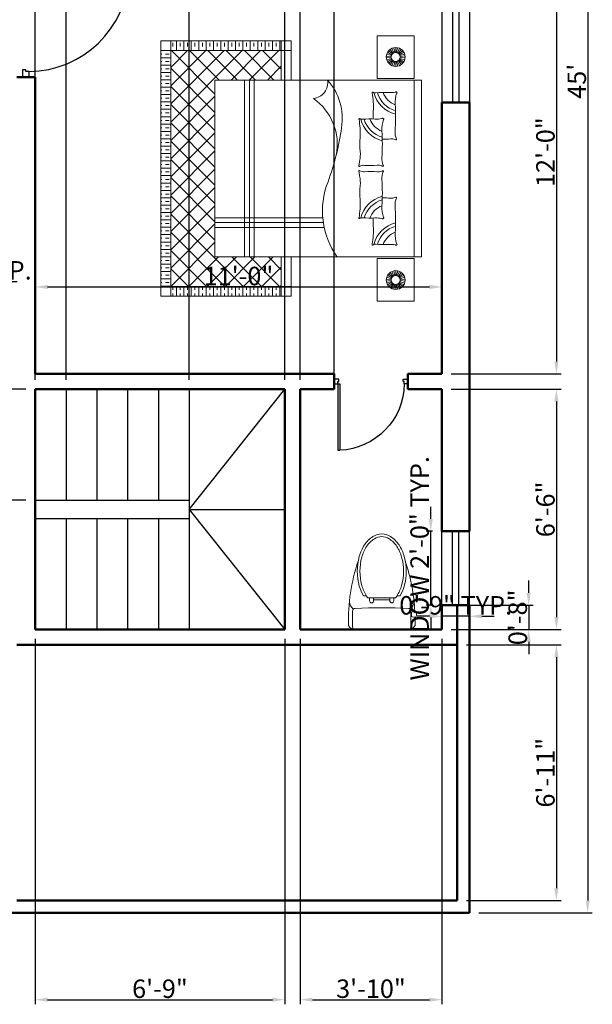
# Model space of a CAD drawing. Units: inches. Extents: x 749 to 1130, y 885 to 1490.
# Tile 2 of 5: x 944 to 1130, y 885 to 1204. Entities that reach past the tile are written whole.
import ezdxf

# ---------------------------------------------------------------- set-up
doc = ezdxf.new("R2010")
doc.units = ezdxf.units.IN
doc.header["$MEASUREMENT"] = 0
for name, color, linetype, lineweight in [('A-ANNO-DIMS', 2, 'Continuous', 18), ('A-DOOR', 2, 'Continuous', 25), ('A-FLOR-FIXT', 9, 'Continuous', 20), ('A-FLOR-STRS', 7, 'Continuous', 25), ('A-FURN', 9, 'Continuous', 18), ('WALL', 7, 'Continuous', 50), ('WINDOW', 2, 'Continuous', 25)]:
    doc.layers.add(name, color=color, linetype=linetype, lineweight=lineweight)
doc.styles.get("Standard").update_dxf_attribs({"font": 'arial.ttf'})
doc.dimstyles.new('yqi0', dxfattribs={"dimscale": 0, "dimtxt": 6, "dimasz": 4, "dimexe": 1.5, "dimexo": 3, "dimgap": 0.5, "dimtad": 1, "dimdsep": 46, "dimlunit": 4, "dimtxsty": 'Standard', "dimcen": 0, "dimclrd": 256, "dimclre": 256, "dimclrt": 7, "dimadec": 1, "dimazin": 2, "dimtfac": 1, "dimtix": 1, "dimtmove": 2, "dimatfit": 2, "dimfxl": 1, "dimtolj": 1, "dimtzin": 0, "dimarcsym": 0})

# ---------------------------------------------------------------- blocks, each defined once
blk = doc.blocks.new('*D3')
at = {"layer": 'A-ANNO-DIMS', "color": 0, "lineweight": -2, "transparency": 16777216}
for p, q in [((1093.07, 1454.46), (1129.93, 1454.46)), ((1128.43, 1450.46), (1128.43, 918.46)), ((1093.07, 914.46), (1129.93, 914.46))]:
    blk.add_line(p, q, dxfattribs=at)
at = {"layer": 'A-ANNO-DIMS', "color": 0, "transparency": 16777216}
for points in [[(1127.76, 1450.46), (1129.09, 1450.46), (1128.43, 1454.46)], [(1127.76, 918.46), (1129.09, 918.46), (1128.43, 914.46)]]:
    blk.add_solid(points, dxfattribs=at)
at = {"layer": 'Defpoints', "color": 0, "transparency": 16777216}
for p in [(1090.07, 1454.46), (1090.07, 914.46), (1128.43, 914.46)]:
    blk.add_point(p, dxfattribs=at)
at = {"layer": 'A-ANNO-DIMS', "color": 0, "transparency": 16777216, "insert": (1124.88, 1184.46), "char_height": 6, "attachment_point": 5, "rotation": 90}
blk.add_mtext("\\A1;45'", dxfattribs=at)
blk = doc.blocks.new('WD_WIN4')
for p, q in [((-0.5, 0.5), (0.5, 0.5)), ((-0.5, 0.12), (0.5, 0.12)), ((-0.5, -0.12), (0.5, -0.12)), ((-0.5, -0.5), (0.5, -0.5))]:
    blk.add_line(p, q)
blk = doc.blocks.new('DR_D01')
for p, q in [((-0.45, 0.93), (-0.42, 0.93)), ((-0.45, 0.03), (-0.45, 0.93)), ((-0.42, 0.03), (-0.42, 0.93)), ((-0.5, 0.03), (-0.42, 0.03)), ((-0.5, 0.03), (-0.5, -0.03)), ((-0.45, 0.03), (-0.45, 0)), ((-0.45, 0), (-0.435, 0)), ((-0.435, 0), (-0.435, -0.03)), ((0.435, 0), (0.435, -0.03)), ((0.45, 0), (0.435, 0)), ((0.45, 0.03), (0.45, 0)), ((0.5, 0.03), (0.45, 0.03)), ((0.5, -0.03), (0.5, 0.03)), ((-0.435, -0.03), (-0.5, -0.03)), ((0.435, -0.03), (0.5, -0.03))]:
    blk.add_line(p, q)
blk.add_arc((-0.4602, 0.0206), 0.9103, 0.59152, 87.46644)
blk = doc.blocks.new('yq_matong_01')
for p, q in [((0, 200.5), (0, -200.5)), ((20, 220.5), (138.8, 220.5)), ((215.8, 91), (238, 91)), ((238, 104.1), (238, -104.1)), ((252.5, 138), (252.5, 114.5)), ((215.8, 61), (238, 61)), ((223, 61), (223, -61)), ((215.8, -61), (238, -61)), ((215.8, -91), (238, -91)), ((252.5, -114.5), (252.5, -138)), ((20, -220.5), (138.8, -220.5)), ((97.4, -220.5), (97.4, -225.5)), ((131.6, -220.5), (131.6, -225.5)), ((97.4, -225.5), (131.6, -225.5))]:
    blk.add_line(p, q)
for centre, radius, start, end in [((54.8, 202.4), 54.8, 117.32201, 181.89921), ((63.9, -1165.4), 1416.8, 71.40679, 91.38565), ((216.6, 161.2), 83.2, 95.49628, 139.93242), ((20, 200.5), 20, 90, 180), ((138.8, 200.5), 20, 2.30634, 90), ((-4840.4, 0), 5003.3, 357.69366, 2.30634), ((406.6, -122.9), 283, 105.20877, 123.27785), ((406.6, -122.9), 303, 105.20877, 120.56985), ((439, -242.2), 426.7, 74.79123, 105.20877), ((439, -242.2), 406.7, 74.79123, 105.20877), ((471.4, -122.9), 283, 56.72215, 74.79123), ((471.4, -122.9), 303, 56.72215, 74.79123), ((215.8, 76), 15, 90, 270), ((357.1, -47.5), 192.8, 123.27785, 128.13838), ((520.9, -47.5), 192.8, 32.25649, 56.72215), ((520.9, -47.5), 212.8, 32.25649, 56.72215), ((596.2, 0), 103.8, 360, 32.25649), ((596.2, 0), 123.8, 360, 32.25649), ((215.8, -76), 15, 90, 270), ((520.9, 47.5), 192.8, 303.27785, 327.74351), ((520.9, 47.5), 212.8, 303.27785, 327.74351), ((596.2, 0), 103.8, 327.74351, 360), ((596.2, 0), 123.8, 327.74351, 360), ((357.1, 47.5), 192.8, 231.86162, 236.72215), ((406.6, 122.9), 283, 236.72215, 254.79123), ((406.6, 122.9), 303, 239.43015, 254.79123), ((471.4, 122.9), 283, 285.20877, 303.27785), ((471.4, 122.9), 303, 285.20877, 303.27785), ((51.3, -204.4), 51.4, 175.68696, 245.09182), ((20, -200.5), 20, 180, 270), ((63.9, 1165.4), 1416.8, 272.89667, 288.59321), ((138.8, -200.5), 20, 270, 357.69366), ((216.6, -161.2), 83.2, 220.06758, 264.50372), ((439, 242.2), 426.7, 254.79123, 285.20877), ((439, 242.2), 406.7, 254.79123, 285.20877), ((63.9, 1165.4), 1416.8, 268.61435, 271.20362), ((156.6, -247.4), 63.1, 159.68336, 188.49388), ((114.1, -225.6), 37, 237.52867, 304.27722), ((72.4, -247.4), 63.1, 352.09441, 20.31664)]:
    blk.add_arc(centre, radius, start, end)
blk = doc.blocks.new('BED')
h = blk.add_hatch()
h.set_pattern_fill('TRANS', color=256, scale=12, style=0)
h.set_pattern_definition([(360, (4433.967, -9715.0492), (1e-15, 3), []), (360, (4433.967, -9713.5492), (1e-15, 3), [1.5, -1.5])])
h.paths.add_polyline_path([(48, -103), (52, -103), (52, -58), (48, -58)])
h.paths.add_polyline_path([(-48, -58), (-52, -58), (-52, -103), (-48, -103)])
h = blk.add_hatch()
h.set_pattern_fill('ANSI37', color=256, scale=42, angle=-90, style=0)
h.set_pattern_definition([(315, (7787.1367, 4477.8466), (3.7123106, 3.7123106), []), (45, (7787.1367, 4477.8466), (-3.7123106, 3.7123106), [])])
h.paths.add_polyline_path([(-36, -85), (-36, -58), (-48, -58), (-48, -103), (48, -103), (48, -58), (36, -58), (36, -85)])
h = blk.add_hatch()
h.set_pattern_fill('TRANS', color=256, scale=12, angle=-90, style=0)
h.set_pattern_definition([(270, (4433.967, -9715.0492), (3, -1e-15), []), (270, (4435.467, -9715.0492), (3, -1e-15), [1.5, -1.5])])
h.paths.add_polyline_path([(48, -107), (48, -103), (-48, -103), (-48, -107)])
for p, q in [((-54, -4), (-54, -19)), ((-36.64, -4), (-54, -4)), ((-36.64, -4), (-36.64, -19)), ((-36, -1), (36, -1)), ((-36, -85), (-36, -1)), ((-36, -4), (36, -4)), ((36, -1), (36, -85)), ((36.64, -4), (36.64, -19)), ((36.64, -4), (54, -4)), ((54, -4), (54, -19)), ((-45.96, -9.7), (-46.58, -7.8)), ((-45.58, -9.62), (-45.8, -7.63)), ((-45.2, -9.62), (-45, -7.63)), ((-44.82, -9.7), (-44.21, -7.79)), ((44.82, -9.7), (44.21, -7.79)), ((45.2, -9.62), (45, -7.63)), ((45.58, -9.62), (45.8, -7.63)), ((45.96, -9.7), (46.58, -7.8)), ((-47.23, -11.45), (-49.23, -11.45)), ((-47.19, -11.07), (-49.14, -10.66)), ((-47.19, -11.83), (-49.14, -12.25)), ((-47.07, -10.7), (-48.9, -9.89)), ((-46.88, -10.37), (-48.5, -9.2)), ((-46.62, -10.08), (-47.96, -8.6)), ((-46.31, -9.86), (-47.31, -8.13)), ((-44.47, -9.85), (-43.48, -8.12)), ((-44.16, -10.08), (-42.83, -8.59)), ((-43.9, -10.36), (-42.29, -9.18)), ((-43.71, -10.7), (-41.89, -9.88)), ((-43.59, -11.06), (-41.64, -10.64)), ((-43.59, -11.83), (-41.63, -12.24)), ((-43.55, -11.44), (-41.55, -11.44)), ((43.55, -11.44), (41.55, -11.44)), ((43.59, -11.83), (41.63, -12.24)), ((43.59, -11.06), (41.64, -10.64)), ((43.71, -10.7), (41.89, -9.88)), ((43.9, -10.36), (42.29, -9.18)), ((44.16, -10.08), (42.83, -8.59)), ((44.47, -9.85), (43.48, -8.12)), ((46.31, -9.86), (47.31, -8.13)), ((46.62, -10.08), (47.96, -8.6)), ((46.88, -10.37), (48.5, -9.2)), ((47.07, -10.7), (48.9, -9.89)), ((47.19, -11.07), (49.14, -10.66)), ((47.19, -11.83), (49.14, -12.25)), ((47.23, -11.45), (49.23, -11.45)), ((-47.07, -12.2), (-48.89, -13.01)), ((-46.87, -12.53), (-48.49, -13.71)), ((-46.62, -12.81), (-47.95, -14.3)), ((-46.3, -13.04), (-47.3, -14.77)), ((-45.95, -13.2), (-46.57, -15.1)), ((-45.58, -13.27), (-45.78, -15.26)), ((-45.19, -13.27), (-44.98, -15.26)), ((-44.82, -13.19), (-44.2, -15.09)), ((-44.47, -13.04), (-43.46, -14.77)), ((-44.16, -12.81), (-42.82, -14.29)), ((-43.9, -12.52), (-42.28, -13.7)), ((-43.71, -12.19), (-41.88, -13)), ((43.71, -12.19), (41.88, -13)), ((43.9, -12.52), (42.28, -13.7)), ((44.16, -12.81), (42.82, -14.29)), ((44.47, -13.04), (43.46, -14.77)), ((44.82, -13.19), (44.2, -15.09)), ((45.19, -13.27), (44.98, -15.26)), ((45.58, -13.27), (45.78, -15.26)), ((45.95, -13.2), (46.57, -15.1)), ((46.3, -13.04), (47.3, -14.77)), ((46.62, -12.81), (47.95, -14.3)), ((46.87, -12.53), (48.49, -13.71)), ((47.07, -12.2), (48.89, -13.01)), ((-36.64, -19), (-54, -19)), ((36.64, -19), (54, -19)), ((20, -85), (20, -41.14)), ((22, -85), (22, -40.91)), ((24, -85), (24, -40.55)), ((-52, -54), (-52, -107)), ((-52, -54), (-36, -54)), ((-48, -54), (-48, -107)), ((36, -54), (52, -54)), ((48, -54), (48, -107)), ((52, -54), (52, -107)), ((-52, -58), (-36, -58)), ((36, -58), (52, -58)), ((36, -69), (-36, -69)), ((36, -71), (-36, -71)), ((36, -73), (-36, -73)), ((36, -85), (-36, -85)), ((-52, -103), (52, -103)), ((-52, -107), (52, -107))]:
    blk.add_line(p, q)
for centre, radius in [((-45.39, -11.45), 3.84), ((45.39, -11.45), 3.84), ((-45.39, -11.45), 1.84), ((45.39, -11.45), 1.84)]:
    blk.add_circle(centre, radius)
for centre, radius, start, end in [((-30.92, -11.24), 0.328, 35.8976, 208.6272), ((-42.38, -17.5), 12.73, 27.1629, 28.6272), ((-44.37, -13.89), 13.5, 357.4804, 9.3956), ((-33.8, -8.61), 8.46, 289.8695, 338.9843), ((-33.8, -8.61), 12.06, 283.8498, 346.0842), ((-33.8, -8.61), 10.71, 286.0319, 344.1205), ((-26.84, 0.13), 11.82, 251.1782, 273.3982), ((-20.92, -99.64), 88.13, 86.2964, 93.3982), ((-14.79, -4.98), 6.73, 266.2964, 294.303), ((-8.24, -13.16), 3.86, 159.0146, 186.273), ((-11.92, -11.33), 0.242, 335.7259, 114.303), ((-5.69, -14.14), 6.59, 155.7259, 159.0146), ((11.92, -11.33), 0.242, 65.697, 204.2741), ((5.69, -14.14), 6.59, 20.9854, 24.2741), ((8.24, -13.16), 3.86, 353.727, 20.9854), ((14.79, -4.98), 6.73, 245.697, 273.7036), ((20.92, -99.64), 88.13, 86.6018, 93.7036), ((33.8, -8.61), 12.06, 193.9158, 256.1502), ((33.8, -8.61), 10.71, 195.8795, 253.9681), ((33.8, -8.61), 8.46, 201.0157, 250.1305), ((26.84, 0.13), 11.82, 266.6018, 288.8218), ((30.92, -11.24), 0.328, 331.3728, 144.1024), ((44.37, -13.89), 13.5, 170.6044, 182.5196), ((42.38, -17.5), 12.73, 151.3728, 152.8371), ((10.15, -16.29), 41.07, 177.4804, 184.5075), ((-36.64, -16.28), 24.71, 358.5721, 6.273), ((36.64, -16.28), 24.71, 173.727, 181.4279), ((-10.15, -16.29), 41.07, 355.4925, 2.5196), ((-32.67, -19.67), 1.88, 339.2246, 4.5075), ((-20.16, -16.62), 0.328, 35.8976, 208.6272), ((-31.62, -22.87), 12.73, 27.1629, 28.6272), ((-33.61, -19.26), 13.5, 357.4804, 9.3956), ((-23.04, -13.99), 8.46, 289.8695, 338.9843), ((20.91, -21.66), 41.07, 177.4804, 184.5075), ((-23.04, -13.99), 12.06, 283.8498, 346.0842), ((-23.04, -13.99), 10.71, 286.0319, 344.1205), ((-16.08, -5.24), 11.82, 251.1782, 273.3982), ((-10.15, -105.01), 88.13, 86.2964, 93.3982), ((-4.03, -10.35), 6.73, 266.2964, 294.303), ((2.52, -18.53), 3.86, 159.0146, 186.273), ((-25.88, -21.66), 24.71, 354.3784, 6.273), ((-1.16, -16.7), 0.242, 335.7259, 114.303), ((5.07, -19.51), 6.59, 155.7259, 159.0146), ((1.16, -16.7), 0.242, 65.697, 204.2741), ((-5.07, -19.51), 6.59, 20.9854, 24.2741), ((-2.52, -18.53), 3.86, 353.727, 20.9854), ((25.88, -21.66), 24.71, 173.727, 185.6216), ((4.03, -10.35), 6.73, 245.697, 273.7036), ((10.15, -105.01), 88.13, 86.6018, 93.7036), ((23.04, -13.99), 12.06, 193.9158, 256.1502), ((23.04, -13.99), 10.71, 195.8795, 253.9681), ((23.04, -13.99), 8.46, 201.0157, 250.1305), ((16.08, -5.24), 11.82, 266.6018, 288.8218), ((20.16, -16.62), 0.328, 331.3728, 144.1024), ((-20.91, -21.66), 41.07, 355.4925, 2.5196), ((33.61, -19.26), 13.5, 170.6044, 182.5196), ((31.62, -22.87), 12.73, 151.3728, 152.8371), ((32.67, -19.67), 1.88, 175.4925, 200.7754), ((-30.88, -20.82), 0.25, 147.6219, 311.9343), ((-32.72, -19.65), 1.93, 327.6219, 339.2246), ((-25.16, -53.53), 33, 93.5164, 99.6766), ((-25.27, -51.86), 31.33, 86.4836, 93.5164), ((-21.12, 15.68), 36.34, 266.4836, 271.5234), ((21.12, 15.68), 36.34, 268.4766, 273.5164), ((25.27, -51.86), 31.33, 86.4836, 93.5164), ((25.16, -53.53), 33, 80.3234, 86.4836), ((30.88, -20.82), 0.25, 228.0657, 32.3781), ((32.72, -19.65), 1.93, 200.7754, 212.3781), ((-20.12, -26.19), 0.25, 147.6219, 311.9343), ((-21.96, -25.02), 1.93, 327.6219, 339.2246), ((-21.91, -25.04), 1.88, 339.2246, 4.5075), ((-14.4, -58.9), 33, 93.5164, 99.6766), ((-14.51, -57.23), 31.33, 86.4836, 93.5164), ((-10.35, 10.3), 36.34, 266.4836, 275.306), ((-5.78, -38.98), 13.15, 77.9645, 95.306), ((2.5, -0.17), 26.53, 257.9645, 261.9243), ((2.55, -24.46), 3.86, 174.3784, 204.7617), ((-1.09, -26.25), 0.228, 231.9005, 52.8902), ((1.09, -26.25), 0.228, 127.1098, 308.0995), ((-2.55, -24.46), 3.86, 335.2383, 5.6216), ((-2.5, -0.17), 26.53, 278.0757, 282.0355), ((5.78, -38.98), 13.15, 84.694, 102.0355), ((10.35, 10.3), 36.34, 264.694, 273.5164), ((14.51, -57.23), 31.33, 86.4836, 93.5164), ((14.4, -58.9), 33, 80.3234, 86.4836), ((20.12, -26.19), 0.25, 228.0657, 32.3781), ((21.91, -25.04), 1.88, 175.4925, 200.7754), ((21.96, -25.02), 1.93, 200.7754, 212.3781), ((-20.27, -56.85), 23.66, 81.0857, 131.6581), ((-9.91, -57.83), 22.61, 78.6456, 145.1521), ((-32.56, -143.87), 111.55, 70.0977, 81.7735), ((17.27, -9.21), 32.05, 248.2778, 305.7663), ((-34.97, -45.63), 6.55, 6.3172, 99.0807)]:
    blk.add_arc(centre, radius, start, end)
blk = doc.blocks.new('*D15')
at = {"layer": 'A-ANNO-DIMS', "lineweight": -2, "transparency": 16777216}
for p, q in [((1077.47, 1042.33), (1077.47, 1046.33)), ((1078.07, 1038.33), (1075.97, 1038.33)), ((1077.47, 1014.33), (1077.47, 1038.33)), ((1078.07, 1014.33), (1075.97, 1014.33)), ((1077.47, 1010.33), (1077.47, 1006.33))]:
    blk.add_line(p, q, dxfattribs=at)
at = {"layer": 'A-ANNO-DIMS', "transparency": 16777216}
for points in [[(1076.8, 1042.33), (1078.14, 1042.33), (1077.47, 1038.33)], [(1076.8, 1010.33), (1078.14, 1010.33), (1077.47, 1014.33)]]:
    blk.add_solid(points, dxfattribs=at)
at = {"layer": 'Defpoints', "color": 0, "transparency": 16777216}
for p in [(1077.47, 1038.33), (1081.07, 1038.33), (1081.07, 1014.33)]:
    blk.add_point(p, dxfattribs=at)
at = {"layer": 'A-ANNO-DIMS', "color": 7, "transparency": 16777216, "insert": (1073.87, 1026.33), "char_height": 6, "attachment_point": 5, "rotation": 90}
blk.add_mtext('\\A1;WINDOW 2\'-0" TYP.', dxfattribs=at)
blk = doc.blocks.new('*D16')
at = {"layer": 'A-ANNO-DIMS', "lineweight": -2, "transparency": 16777216}
for p, q in [((1077.07, 1010.73), (1073.07, 1010.73)), ((1081.07, 1011.33), (1081.07, 1009.23)), ((1090.07, 1010.73), (1081.07, 1010.73)), ((1090.07, 1011.33), (1090.07, 1009.23)), ((1094.07, 1010.73), (1098.07, 1010.73))]:
    blk.add_line(p, q, dxfattribs=at)
at = {"layer": 'A-ANNO-DIMS', "transparency": 16777216}
for points in [[(1077.07, 1011.4), (1077.07, 1010.07), (1081.07, 1010.73)], [(1094.07, 1011.4), (1094.07, 1010.07), (1090.07, 1010.73)]]:
    blk.add_solid(points, dxfattribs=at)
at = {"layer": 'Defpoints', "color": 0, "transparency": 16777216}
for p in [(1081.07, 1014.33), (1090.07, 1014.33), (1081.07, 1010.73)]:
    blk.add_point(p, dxfattribs=at)
at = {"layer": 'A-ANNO-DIMS', "color": 7, "transparency": 16777216, "insert": (1085.57, 1014.3), "char_height": 6, "attachment_point": 5}
blk.add_mtext('\\A1;0\'-9" TYP.', dxfattribs=at)
blk = doc.blocks.new('*D17')
at = {"layer": 'A-ANNO-DIMS', "lineweight": -2, "transparency": 16777216}
for p, q in [((895.2, 1119.47), (891.2, 1119.47)), ((899.2, 1121.87), (899.2, 1117.97)), ((935.2, 1119.47), (899.2, 1119.47)), ((935.2, 1121.87), (935.2, 1117.97)), ((939.2, 1119.47), (943.2, 1119.47))]:
    blk.add_line(p, q, dxfattribs=at)
at = {"layer": 'A-ANNO-DIMS', "transparency": 16777216}
for points in [[(895.2, 1120.13), (895.2, 1118.8), (899.2, 1119.47)], [(939.2, 1120.13), (939.2, 1118.8), (935.2, 1119.47)]]:
    blk.add_solid(points, dxfattribs=at)
at = {"layer": 'Defpoints', "color": 0, "transparency": 16777216}
for p in [(899.2, 1124.87), (935.2, 1124.87), (899.2, 1119.47)]:
    blk.add_point(p, dxfattribs=at)
at = {"layer": 'A-ANNO-DIMS', "color": 7, "transparency": 16777216, "insert": (917.2, 1123.07), "char_height": 6, "attachment_point": 5}
blk.add_mtext('\\A1;DOOR 3\'-0" TYP.', dxfattribs=at)
blk = doc.blocks.new('*D38')
at = {"layer": 'A-ANNO-DIMS', "lineweight": -2, "transparency": 16777216}
for p, q in [((1084.07, 1233.46), (1119.77, 1233.46)), ((1118.27, 1229.46), (1118.27, 1093.46)), ((1084.07, 1089.46), (1119.77, 1089.46))]:
    blk.add_line(p, q, dxfattribs=at)
at = {"layer": 'A-ANNO-DIMS', "transparency": 16777216}
for points in [[(1117.6, 1229.46), (1118.94, 1229.46), (1118.27, 1233.46)], [(1117.6, 1093.46), (1118.94, 1093.46), (1118.27, 1089.46)]]:
    blk.add_solid(points, dxfattribs=at)
at = {"layer": 'Defpoints', "color": 0, "transparency": 16777216}
for p in [(1081.07, 1233.46), (1081.07, 1089.46), (1118.27, 1089.46)]:
    blk.add_point(p, dxfattribs=at)
at = {"layer": 'A-ANNO-DIMS', "color": 7, "transparency": 16777216, "insert": (1114.71, 1161.46), "char_height": 6, "attachment_point": 5, "rotation": 90}
blk.add_mtext('\\A1;12\'-0"', dxfattribs=at)
blk = doc.blocks.new('*D39')
at = {"layer": 'A-ANNO-DIMS', "lineweight": -2, "transparency": 16777216}
for p, q in [((1084.07, 1084.46), (1119.77, 1084.46)), ((1118.27, 1080.46), (1118.27, 1010.46)), ((1084.07, 1006.46), (1119.77, 1006.46))]:
    blk.add_line(p, q, dxfattribs=at)
at = {"layer": 'A-ANNO-DIMS', "transparency": 16777216}
for points in [[(1117.6, 1080.46), (1118.94, 1080.46), (1118.27, 1084.46)], [(1117.6, 1010.46), (1118.94, 1010.46), (1118.27, 1006.46)]]:
    blk.add_solid(points, dxfattribs=at)
at = {"layer": 'Defpoints', "color": 0, "transparency": 16777216}
for p in [(1081.07, 1084.46), (1081.07, 1006.46), (1118.27, 1006.46)]:
    blk.add_point(p, dxfattribs=at)
at = {"layer": 'A-ANNO-DIMS', "color": 7, "transparency": 16777216, "insert": (1114.71, 1045.46), "char_height": 6, "attachment_point": 5, "rotation": 90}
blk.add_mtext('\\A1;6\'-6"', dxfattribs=at)
blk = doc.blocks.new('*D40')
at = {"layer": 'A-ANNO-DIMS', "lineweight": -2, "transparency": 16777216}
for p, q in [((1089.07, 1001.46), (1119.77, 1001.46)), ((1118.27, 997.46), (1118.27, 922.46)), ((1089.07, 918.46), (1119.77, 918.46))]:
    blk.add_line(p, q, dxfattribs=at)
at = {"layer": 'A-ANNO-DIMS', "transparency": 16777216}
for points in [[(1117.6, 997.46), (1118.94, 997.46), (1118.27, 1001.46)], [(1117.6, 922.46), (1118.94, 922.46), (1118.27, 918.46)]]:
    blk.add_solid(points, dxfattribs=at)
at = {"layer": 'Defpoints', "color": 0, "transparency": 16777216}
for p in [(1086.07, 1001.46), (1086.07, 918.46), (1118.27, 918.46)]:
    blk.add_point(p, dxfattribs=at)
at = {"layer": 'A-ANNO-DIMS', "color": 7, "transparency": 16777216, "insert": (1114.71, 959.96), "char_height": 6, "attachment_point": 5, "rotation": 90}
blk.add_mtext('\\A1;6\'-11"', dxfattribs=at)
blk = doc.blocks.new('*D45')
at = {"layer": 'A-ANNO-DIMS', "lineweight": -2, "transparency": 16777216}
for p, q in [((949.07, 1003.46), (949.07, 884.76)), ((1030.07, 1003.46), (1030.07, 884.76)), ((953.07, 886.26), (1026.07, 886.26))]:
    blk.add_line(p, q, dxfattribs=at)
at = {"layer": 'A-ANNO-DIMS', "transparency": 16777216}
for points in [[(953.07, 886.93), (953.07, 885.59), (949.07, 886.26)], [(1026.07, 886.93), (1026.07, 885.59), (1030.07, 886.26)]]:
    blk.add_solid(points, dxfattribs=at)
at = {"layer": 'Defpoints', "color": 0, "transparency": 16777216}
for p in [(949.07, 1006.46), (1030.07, 1006.46), (1030.07, 886.26)]:
    blk.add_point(p, dxfattribs=at)
at = {"layer": 'A-ANNO-DIMS', "color": 7, "transparency": 16777216, "insert": (989.57, 889.82), "char_height": 6, "attachment_point": 5}
blk.add_mtext('\\A1;6\'-9"', dxfattribs=at)
blk = doc.blocks.new('*D46')
at = {"layer": 'A-ANNO-DIMS', "lineweight": -2, "transparency": 16777216}
for p, q in [((1035.07, 1003.46), (1035.07, 884.76)), ((1081.07, 1003.46), (1081.07, 884.76)), ((1039.07, 886.26), (1077.07, 886.26))]:
    blk.add_line(p, q, dxfattribs=at)
at = {"layer": 'A-ANNO-DIMS', "transparency": 16777216}
for points in [[(1039.07, 886.93), (1039.07, 885.59), (1035.07, 886.26)], [(1077.07, 886.93), (1077.07, 885.59), (1081.07, 886.26)]]:
    blk.add_solid(points, dxfattribs=at)
at = {"layer": 'Defpoints', "color": 0, "transparency": 16777216}
for p in [(1035.07, 1006.46), (1081.07, 1006.46), (1081.07, 886.26)]:
    blk.add_point(p, dxfattribs=at)
at = {"layer": 'A-ANNO-DIMS', "color": 7, "transparency": 16777216, "insert": (1058.07, 889.83), "char_height": 6, "attachment_point": 5}
blk.add_mtext('\\A1;3\'-10"', dxfattribs=at)
blk = doc.blocks.new('*D47')
at = {"layer": 'A-ANNO-DIMS', "lineweight": -2, "transparency": 16777216}
for p, q in [((949.07, 1087.46), (949.07, 1484.16)), ((959.07, 1087.46), (959.07, 1484.16)), ((945.07, 1482.66), (941.07, 1482.66)), ((949.07, 1482.66), (959.07, 1482.66)), ((963.07, 1482.66), (967.07, 1482.66))]:
    blk.add_line(p, q, dxfattribs=at)
at = {"layer": 'A-ANNO-DIMS', "transparency": 16777216}
for points in [[(945.07, 1483.33), (945.07, 1481.99), (949.07, 1482.66)], [(963.07, 1483.33), (963.07, 1481.99), (959.07, 1482.66)]]:
    blk.add_solid(points, dxfattribs=at)
at = {"layer": 'Defpoints', "color": 0, "transparency": 16777216}
for p in [(959.07, 1482.66), (949.07, 1084.46), (959.07, 1084.46)]:
    blk.add_point(p, dxfattribs=at)
at = {"layer": 'A-ANNO-DIMS', "color": 7, "transparency": 16777216, "insert": (954.07, 1486.22), "char_height": 6, "attachment_point": 5}
blk.add_mtext('\\A1;0\'-10"', dxfattribs=at)
blk = doc.blocks.new('*D48')
at = {"layer": 'A-ANNO-DIMS', "lineweight": -2, "transparency": 16777216}
for p, q in [((999.07, 1087.46), (999.07, 1484.16)), ((1030.07, 1087.46), (1030.07, 1484.16)), ((1003.07, 1482.66), (1026.07, 1482.66))]:
    blk.add_line(p, q, dxfattribs=at)
at = {"layer": 'A-ANNO-DIMS', "transparency": 16777216}
for points in [[(1003.07, 1483.33), (1003.07, 1481.99), (999.07, 1482.66)], [(1026.07, 1483.33), (1026.07, 1481.99), (1030.07, 1482.66)]]:
    blk.add_solid(points, dxfattribs=at)
at = {"layer": 'Defpoints', "color": 0, "transparency": 16777216}
for p in [(1030.07, 1482.66), (999.07, 1084.46), (1030.07, 1084.46)]:
    blk.add_point(p, dxfattribs=at)
at = {"layer": 'A-ANNO-DIMS', "color": 7, "transparency": 16777216, "insert": (1014.57, 1486.17), "char_height": 6, "attachment_point": 5}
blk.add_mtext('\\A1;2\'-7"', dxfattribs=at)
blk = doc.blocks.new('*D49')
at = {"layer": 'A-ANNO-DIMS', "lineweight": -2, "transparency": 16777216}
for p, q in [((946.07, 1084.46), (760.37, 1084.46)), ((761.87, 1080.46), (761.87, 1052.46)), ((946.07, 1048.46), (760.37, 1048.46))]:
    blk.add_line(p, q, dxfattribs=at)
at = {"layer": 'A-ANNO-DIMS', "transparency": 16777216}
for points in [[(761.2, 1080.46), (762.54, 1080.46), (761.87, 1084.46)], [(761.2, 1052.46), (762.54, 1052.46), (761.87, 1048.46)]]:
    blk.add_solid(points, dxfattribs=at)
at = {"layer": 'Defpoints', "color": 0, "transparency": 16777216}
for p in [(949.07, 1084.46), (761.87, 1048.46), (949.07, 1048.46)]:
    blk.add_point(p, dxfattribs=at)
at = {"layer": 'A-ANNO-DIMS', "color": 7, "transparency": 16777216, "insert": (758.3, 1066.46), "char_height": 6, "attachment_point": 5, "rotation": 90}
blk.add_mtext('\\A1;3\'-0"', dxfattribs=at)
blk = doc.blocks.new('*D50')
at = {"layer": 'A-ANNO-DIMS', "lineweight": -2, "transparency": 16777216}
for p, q in [((1035.07, 1087.46), (1035.07, 1484.16)), ((1046.07, 1087.46), (1046.07, 1484.16)), ((1031.07, 1482.66), (1027.07, 1482.66)), ((1046.07, 1482.66), (1035.07, 1482.66)), ((1050.07, 1482.66), (1054.07, 1482.66))]:
    blk.add_line(p, q, dxfattribs=at)
at = {"layer": 'A-ANNO-DIMS', "transparency": 16777216}
for points in [[(1031.07, 1483.33), (1031.07, 1481.99), (1035.07, 1482.66)], [(1050.07, 1483.33), (1050.07, 1481.99), (1046.07, 1482.66)]]:
    blk.add_solid(points, dxfattribs=at)
at = {"layer": 'Defpoints', "color": 0, "transparency": 16777216}
for p in [(1035.07, 1482.66), (1035.07, 1084.46), (1046.07, 1084.46)]:
    blk.add_point(p, dxfattribs=at)
at = {"layer": 'A-ANNO-DIMS', "color": 7, "transparency": 16777216, "insert": (1040.57, 1486.22), "char_height": 6, "attachment_point": 5}
blk.add_mtext('\\A1;0\'-11"', dxfattribs=at)
blk = doc.blocks.new('*D64')
at = {"layer": 'A-ANNO-DIMS', "lineweight": -2, "transparency": 16777216}
for p, q in [((949.07, 1092.46), (949.07, 1119.16)), ((1081.07, 1092.46), (1081.07, 1119.16)), ((953.07, 1117.66), (1077.07, 1117.66))]:
    blk.add_line(p, q, dxfattribs=at)
at = {"layer": 'A-ANNO-DIMS', "transparency": 16777216}
for points in [[(953.07, 1118.33), (953.07, 1116.99), (949.07, 1117.66)], [(1077.07, 1118.33), (1077.07, 1116.99), (1081.07, 1117.66)]]:
    blk.add_solid(points, dxfattribs=at)
at = {"layer": 'Defpoints', "color": 0, "transparency": 16777216}
for p in [(1081.07, 1117.66), (949.07, 1089.46), (1081.07, 1089.46)]:
    blk.add_point(p, dxfattribs=at)
at = {"layer": 'A-ANNO-DIMS', "color": 7, "transparency": 16777216, "insert": (1015.07, 1121.22), "char_height": 6, "attachment_point": 5}
blk.add_mtext('\\A1;11\'-0"', dxfattribs=at)
blk = doc.blocks.new('*D65')
at = {"layer": 'A-ANNO-DIMS', "lineweight": -2, "transparency": 16777216}
for p, q in [((1109.27, 1018.33), (1109.27, 1022.33)), ((1084.07, 1014.33), (1110.77, 1014.33)), ((1109.27, 1014.33), (1109.27, 1006.46)), ((1084.07, 1006.46), (1110.77, 1006.46)), ((1109.27, 1002.46), (1109.27, 998.46))]:
    blk.add_line(p, q, dxfattribs=at)
at = {"layer": 'A-ANNO-DIMS', "transparency": 16777216}
for points in [[(1108.6, 1018.33), (1109.94, 1018.33), (1109.27, 1014.33)], [(1108.6, 1002.46), (1109.94, 1002.46), (1109.27, 1006.46)]]:
    blk.add_solid(points, dxfattribs=at)
at = {"layer": 'Defpoints', "color": 0, "transparency": 16777216}
for p in [(1081.07, 1014.33), (1081.07, 1006.46), (1109.27, 1006.46)]:
    blk.add_point(p, dxfattribs=at)
at = {"layer": 'A-ANNO-DIMS', "color": 7, "transparency": 16777216, "insert": (1105.71, 1010.4), "char_height": 6, "attachment_point": 5, "rotation": 90}
blk.add_mtext('\\A1;0\'-8"', dxfattribs=at)

msp = doc.modelspace()

# ---------------------------------------------------------------- linework, layer by layer
at = {"layer": 'A-FLOR-STRS'}
for p, q in [((959.07, 1084.46), (959.07, 1048.46)), ((969.07, 1084.46), (969.07, 1048.46)), ((979.07, 1084.46), (979.07, 1048.46)), ((989.07, 1084.46), (989.07, 1048.46)), ((999.07, 1084.46), (999.07, 1048.46)), ((999.07, 1045.46), (1030.07, 1084.46)), ((949.07, 1048.46), (999.07, 1048.46)), ((999.07, 1048.46), (999.07, 1042.46)), ((999.07, 1045.46), (1030.07, 1045.46)), ((999.07, 1045.46), (1030.07, 1006.46)), ((949.07, 1042.46), (999.07, 1042.46)), ((959.07, 1042.46), (959.07, 1006.46)), ((969.07, 1042.46), (969.07, 1006.46)), ((979.07, 1042.46), (979.07, 1006.46)), ((989.07, 1042.46), (989.07, 1006.46)), ((999.07, 1042.46), (999.07, 1006.46))]:
    msp.add_line(p, q, dxfattribs=at)
at = {"layer": 'WALL'}
for p, q in [((943.07, 1185.834), (949.07, 1185.834)), ((949.07, 1185.834), (949.07, 1089.46)), ((949.07, 1185.834), (949.07, 1171.334)), ((1081.07, 1089.46), (1081.07, 1177.586)), ((1081.07, 1177.586), (1090.07, 1177.586)), ((1090.07, 1038.334), (1090.07, 1177.586)), ((949.07, 1089.46), (1046.07, 1089.46)), ((1046.07, 1084.46), (1046.07, 1089.46)), ((1070.07, 1089.46), (1081.07, 1089.46)), ((1070.07, 1084.46), (1070.07, 1089.46)), ((949.07, 1084.46), (1030.07, 1084.46)), ((949.07, 1084.46), (949.07, 1083.46)), ((1030.07, 1006.46), (1030.07, 1084.46)), ((1035.07, 1006.46), (1035.07, 1084.46)), ((1035.07, 1084.46), (1046.07, 1084.46)), ((1070.07, 1084.46), (1081.07, 1084.46)), ((1081.07, 1038.334), (1081.07, 1084.46)), ((949.07, 1083.46), (949.07, 1006.46)), ((1081.07, 1038.334), (1090.07, 1038.334)), ((1081.07, 1006.46), (1081.07, 1014.334)), ((1081.07, 1014.334), (1090.07, 1014.334)), ((1086.07, 918.46), (1086.07, 1014.334)), ((1090.07, 914.46), (1090.07, 1014.334)), ((949.07, 1006.46), (1030.07, 1006.46)), ((1035.07, 1006.46), (1081.07, 1006.46)), ((943.07, 1001.46), (1086.07, 1001.46)), ((943.07, 918.46), (1086.07, 918.46)), ((790.07, 914.46), (1090.07, 914.46))]:
    msp.add_line(p, q, dxfattribs=at)

# ---------------------------------------------------------------- block references
at = {"layer": 'A-DOOR', "xscale": -36, "yscale": -36, "zscale": 36, "rotation": 90.00000000000017}
msp.add_blockref('DR_D01', (946.07, 1203.834), dxfattribs=at)
at = {"layer": 'A-DOOR', "xscale": 24, "yscale": -24, "zscale": 24}
msp.add_blockref('DR_D01', (1058.07, 1086.96), dxfattribs=at)
at = {"layer": 'A-FLOR-FIXT', "xscale": 0.0430468521740032, "yscale": 0.0430468521740032, "zscale": 0.0430468521740032, "rotation": 89.99999999999999}
msp.add_blockref('yq_matong_01', (1061.564, 1006.467), dxfattribs=at)
at = {"layer": 'A-FURN', "xscale": 0.797910650636604, "yscale": 0.797910650636604, "zscale": 0.797910650636604, "rotation": 270}
msp.add_blockref('BED', (1075.235, 1156.12), dxfattribs=at)
at = {"layer": 'WINDOW'}
for p, xscale, yscale, zscale, rotation in [((1085.57, 1201.586), 48, 9.000000000001592, 48, 269.9999999999998), ((1085.57, 1026.334), 24, 9.000000000000455, 24, 90)]:
    msp.add_blockref('WD_WIN4', p, dxfattribs=dict(at, xscale=xscale, yscale=yscale, zscale=zscale, rotation=rotation))

# ---------------------------------------------------------------- dimensions: what is measured, and where the dimension line sits
at = {"layer": 'A-ANNO-DIMS'}
for base, p1, p2, picture, middle in [((959.07, 1482.66), (949.07, 1084.46), (959.07, 1084.46), '*D47', (954.07, 1486.224)), ((1030.07, 1482.66), (999.07, 1084.46), (1030.07, 1084.46), '*D48', (1014.57, 1486.173)), ((1035.07, 1482.66), (1046.07, 1084.46), (1035.07, 1084.46), '*D50', (1040.57, 1486.224)), ((1030.07, 886.26), (949.07, 1006.46), (1030.07, 1006.46), '*D45', (989.57, 889.824)), ((1081.07, 886.26), (1035.07, 1006.46), (1081.07, 1006.46), '*D46', (1058.07, 889.826))]:
    dim = msp.add_linear_dim(base=base, p1=p1, p2=p2, dimstyle='yqi0', override={"dimscale": 1, "dimdec": 1, "dimzin": 1, "dimfrac": 2}, dxfattribs=at)
    dim.commit()
    dim.dimension.update_dxf_attribs({"geometry": picture, "text_midpoint": middle})
dim = msp.add_aligned_dim(p1=(1090.07, 1454.46), p2=(1090.07, 914.46), distance=38.358, dimstyle='yqi0', override={"dimscale": 1, "dimclrd": 0, "dimclre": 0, "dimclrt": 0}, dxfattribs=at)
dim.commit()
dim.dimension.update_dxf_attribs({"geometry": '*D3', "text_midpoint": (1124.877, 1184.46)})
for base, p1, p2, angle, picture, middle in [((1118.27, 1089.46), (1081.07, 1233.46), (1081.07, 1089.46), 90, '*D38', (1114.706, 1161.46)), ((1081.07, 1117.66), (949.07, 1089.46), (1081.07, 1089.46), 0, '*D64', (1015.07, 1121.224)), ((761.87, 1048.46), (949.07, 1084.46), (949.07, 1048.46), 90, '*D49', (758.304, 1066.46)), ((1118.27, 1006.46), (1081.07, 1084.46), (1081.07, 1006.46), 90, '*D39', (1114.706, 1045.46)), ((1109.27, 1006.46), (1081.07, 1014.334), (1081.07, 1006.46), 270, '*D65', (1105.706, 1010.397)), ((1118.27, 918.46), (1086.07, 1001.46), (1086.07, 918.46), 90, '*D40', (1114.706, 959.96))]:
    dim = msp.add_linear_dim(base=base, p1=p1, p2=p2, angle=angle, dimstyle='yqi0', override={"dimscale": 1, "dimdec": 1, "dimzin": 1, "dimfrac": 2}, dxfattribs=at)
    dim.commit()
    dim.dimension.update_dxf_attribs({"geometry": picture, "text_midpoint": middle})
for base, p1, p2, angle, text, picture, middle in [((899.202, 1119.465), (935.202, 1124.865), (899.202, 1124.865), 180, 'DOOR <> TYP.', '*D17', (917.202, 1123.072)), ((1077.47, 1038.334), (1081.07, 1014.334), (1081.07, 1038.334), 90, 'WINDOW <> TYP.', '*D15', (1073.866, 1026.334)), ((1081.07, 1010.734), (1090.07, 1014.334), (1081.07, 1014.334), 180, '<> TYP.', '*D16', (1085.57, 1014.298))]:
    dim = msp.add_linear_dim(base=base, p1=p1, p2=p2, angle=angle, text=text, dimstyle='yqi0', override={"dimscale": 1, "dimdec": 1, "dimzin": 1, "dimfrac": 2}, dxfattribs=at)
    dim.commit()
    dim.dimension.update_dxf_attribs({"geometry": picture, "text_midpoint": middle})

doc.saveas('drawing.dxf')
